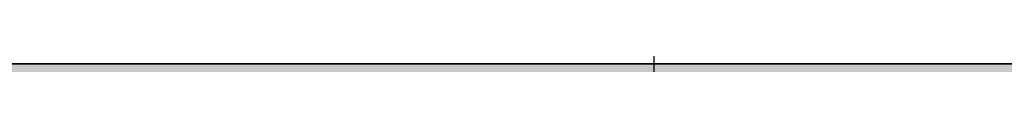
# Model space of a CAD drawing. Units: inches. Extents: x 2083 to 3317, y 1141 to 2115.
# Tile 51 of 256: x 2237.106 to 2238.294, y 1477.761 to 1477.761. Entities that reach past the tile are written whole.
import ezdxf

# ---------------------------------------------------------------- set-up
doc = ezdxf.new("R2010")
doc.units = ezdxf.units.IN
doc.layers.add('A-ANNO-DIMS', color=2, linetype='Continuous', lineweight=18)
doc.layers.add('A-WALL', color=7, linetype='Continuous', lineweight=35)
doc.layers.add('A-WALL-PATT', color=251, linetype='Continuous', lineweight=13, true_color=0x636466)
doc.styles.get("Standard").update_dxf_attribs({"font": 'arial.ttf'})
doc.dimstyles.new('ISO-25', dxfattribs={"dimtxt": 12, "dimasz": 12, "dimexe": 1.25, "dimexo": 0.625, "dimtad": 1, "dimlunit": 3, "dimtxsty": 'Standard', "dimcen": 2.5, "dimadec": 0, "dimazin": 0, "dimtfac": 1, "dimtmove": 0, "dimatfit": 3, "dimfxl": 1, "dimarcsym": 0})

# ---------------------------------------------------------------- blocks, each defined once
blk = doc.blocks.new('*D30')
at = {"layer": 'A-ANNO-DIMS', "color": 0, "lineweight": -2, "transparency": 16777216}
for p, q in [((2240.0179, 1445.2738), (2240.0179, 1448.0455)), ((2254.3293, 1445.2738), (2254.3293, 1448.0455)), ((2228.0179, 1446.7955), (2216.0179, 1446.7955)), ((2240.0179, 1446.7955), (2254.3293, 1446.7955)), ((2266.3293, 1446.7955), (2413.7649, 1446.7955))]:
    blk.add_line(p, q, dxfattribs=at)
at = {"layer": 'A-ANNO-DIMS', "color": 0, "transparency": 16777216}
for points in [[(2228.0179, 1448.7955), (2228.0179, 1444.7955), (2240.0179, 1446.7955)], [(2266.3293, 1448.7955), (2266.3293, 1444.7955), (2254.3293, 1446.7955)]]:
    blk.add_solid(points, dxfattribs=at)
at = {"layer": 'Defpoints', "color": 0, "transparency": 16777216}
for p in [(2254.3293, 1446.7955), (2240.0179, 1444.6488), (2254.3293, 1444.6488)]:
    blk.add_point(p, dxfattribs=at)
at = {"layer": 'A-ANNO-DIMS', "color": 0, "transparency": 16777216, "insert": (2346.0471, 1453.6252), "char_height": 12, "attachment_point": 5}
blk.add_mtext('WC 1\'-2 1/2" TYP.', dxfattribs=at)
blk = doc.blocks.new('*D31')
at = {"layer": 'A-ANNO-DIMS', "color": 0, "lineweight": -2, "transparency": 16777216}
for p, q in [((2237.8711, 1456.6488), (2237.8711, 1541.9152)), ((2239.3929, 1444.6488), (2236.6211, 1444.6488)), ((2237.8711, 1431.5475), (2237.8711, 1444.6488)), ((2239.3929, 1431.5475), (2236.6211, 1431.5475)), ((2237.8711, 1419.5475), (2237.8711, 1407.5475))]:
    blk.add_line(p, q, dxfattribs=at)
at = {"layer": 'A-ANNO-DIMS', "color": 0, "transparency": 16777216}
for points in [[(2235.8711, 1456.6488), (2239.8711, 1456.6488), (2237.8711, 1444.6488)], [(2235.8711, 1419.5475), (2239.8711, 1419.5475), (2237.8711, 1431.5475)]]:
    blk.add_solid(points, dxfattribs=at)
at = {"layer": 'Defpoints', "color": 0, "transparency": 16777216}
for p in [(2237.8711, 1444.6488), (2240.0179, 1444.6488), (2240.0179, 1431.5475)]:
    blk.add_point(p, dxfattribs=at)
at = {"layer": 'A-ANNO-DIMS', "color": 0, "transparency": 16777216, "insert": (2231.2175, 1505.282), "char_height": 12, "attachment_point": 5, "rotation": 90}
blk.add_mtext('1\'-1" TYP.', dxfattribs=at)
blk = doc.blocks.new('*D45')
at = {"layer": 'A-ANNO-DIMS', "color": 0, "lineweight": -2, "transparency": 16777216}
for p, q in [((2235.9598, 1478.3864), (2235.9598, 1531.3614)), ((2418.9598, 1478.3864), (2418.9598, 1531.3614)), ((2247.9598, 1530.1114), (2406.9598, 1530.1114))]:
    blk.add_line(p, q, dxfattribs=at)
at = {"layer": 'A-ANNO-DIMS', "color": 0, "transparency": 16777216}
for points in [[(2247.9598, 1532.1114), (2247.9598, 1528.1114), (2235.9598, 1530.1114)], [(2406.9598, 1532.1114), (2406.9598, 1528.1114), (2418.9598, 1530.1114)]]:
    blk.add_solid(points, dxfattribs=at)
at = {"layer": 'Defpoints', "color": 0, "transparency": 16777216}
for p in [(2418.9598, 1530.1114), (2235.9598, 1477.7614), (2418.9598, 1477.7614)]:
    blk.add_point(p, dxfattribs=at)
at = {"layer": 'A-ANNO-DIMS', "color": 0, "transparency": 16777216, "insert": (2327.4598, 1536.8673), "char_height": 12, "attachment_point": 5}
blk.add_mtext('15\'-3"', dxfattribs=at)
blk = doc.blocks.new('*D62')
at = {"layer": 'A-ANNO-DIMS', "color": 0, "lineweight": -2, "transparency": 16777216}
for p, q in [((2235.9598, 1469.3864), (2235.9598, 1522.3614)), ((2379.9598, 1469.3864), (2379.9598, 1522.3614)), ((2247.9598, 1521.1114), (2367.9598, 1521.1114))]:
    blk.add_line(p, q, dxfattribs=at)
at = {"layer": 'A-ANNO-DIMS', "color": 0, "transparency": 16777216}
for points in [[(2247.9598, 1523.1114), (2247.9598, 1519.1114), (2235.9598, 1521.1114)], [(2367.9598, 1523.1114), (2367.9598, 1519.1114), (2379.9598, 1521.1114)]]:
    blk.add_solid(points, dxfattribs=at)
at = {"layer": 'Defpoints', "color": 0, "transparency": 16777216}
for p in [(2379.9598, 1521.1114), (2235.9598, 1468.7614), (2379.9598, 1468.7614)]:
    blk.add_point(p, dxfattribs=at)
at = {"layer": 'A-ANNO-DIMS', "color": 0, "transparency": 16777216, "insert": (2307.9598, 1527.8632), "char_height": 12, "attachment_point": 5}
blk.add_mtext('12\'-0"', dxfattribs=at)

msp = doc.modelspace()

# ---------------------------------------------------------------- hatches: boundary and pattern name
at = {"layer": 'A-WALL-PATT'}
h = msp.add_hatch(color=256, dxfattribs=at)
h.dxf.hatch_style = 1
h.paths.add_polyline_path([(3126.9598, 2020.7614), (2748.9598, 2020.7614), (2604.9598, 2020.7614), (2226.9598, 2020.7614), (2226.9598, 1702.7614), (2466.9598, 1702.7614), (2466.9598, 1582.7614), (2418.9598, 1582.7614), (2418.9598, 1477.7614), (2226.9598, 1477.7614), (2226.9598, 1263.2614), (2544.9598, 1263.2614), (2544.9598, 1411.7614), (2604.9598, 1411.7614), (2685.9598, 1411.7614), (2685.9598, 1420.7614), (2604.9598, 1420.7614), (2604.9598, 1573.7614), (2604.9598, 1702.7614), (2604.9598, 2011.7614), (2748.9598, 2011.7614), (2748.9598, 1702.7614), (2862.9598, 1702.7614), (2862.9598, 1621.7614), (2871.9598, 1621.7614), (2871.9598, 1702.7614), (2883.9598, 1702.7614), (2883.9598, 1706.9395, -0.026459), (2883.9598, 1711.7614), (2757.9598, 1711.7614), (2757.9598, 1807.7614), (2787.9598, 1807.7614), (2787.9598, 1812.2614), (2757.9598, 1812.2614), (2757.9598, 2011.7614), (2877.9598, 2011.7614), (2877.9598, 1812.2614), (2847.9598, 1812.2614), (2847.9598, 1807.7614), (2889.8357, 1807.7614), (2889.8357, 1812.2614), (2882.4598, 1812.2614), (2882.4598, 2011.7614), (3117.9598, 2011.7614), (3117.9598, 1812.2614), (2937.8357, 1812.2614), (2937.8357, 1807.7614), (2995.7098, 1807.7614), (2995.7098, 1796.1177), (3000.2098, 1796.1177), (3000.2098, 1807.7614), (3117.9598, 1807.7614), (3117.9598, 1711.7614), (3000.2098, 1711.7614), (3000.2098, 1760.1177), (2998.5727, 1760.1177, -0.020711), (2995.7098, 1760.1177), (2995.7098, 1711.7614), (2931.9598, 1711.7614), (2931.9598, 1702.7614), (3126.9598, 1702.7614)])
h.paths.add_polyline_path([(2471.4598, 2011.7614), (2471.4598, 1810.0114), (2462.7169, 1810.0114), (2462.7169, 1805.5114), (2505.9598, 1805.5114), (2505.9598, 1810.0114), (2475.9598, 1810.0114), (2475.9598, 2011.7614), (2595.9598, 2011.7614), (2595.9598, 1810.0114), (2565.9598, 1810.0114), (2565.9598, 1805.5114), (2595.9598, 1805.5114), (2595.9598, 1711.7614), (2235.9598, 1711.7614), (2235.9598, 1805.5114), (2353.7098, 1805.5114), (2353.7098, 1796.0542), (2358.2098, 1796.0542), (2358.2098, 1805.5114), (2414.7169, 1805.5114), (2414.7169, 1810.0114), (2235.9598, 1810.0114), (2235.9598, 2011.7614)], flags=16)
h.paths.add_polyline_path([(2270.2047, 1994.61), (2270.2047, 1970.61), (2246.2047, 1970.61), (2246.2047, 1994.61)], flags=0)
edge = h.paths.add_edge_path(flags=0)
edge.add_ellipse((2332.0274, 1899.7982), major_axis=(-3.043, 3.043), ratio=0.168252, start_angle=-161.3322, end_angle=-156.3071, ccw=False)
edge.add_ellipse((2333.082, 1898.7435), major_axis=(-1.0546, 1.0546), ratio=0.453532, start_angle=-123.371, end_angle=-94.1591)
edge = h.paths.add_edge_path(flags=0)
edge.add_ellipse((2332.0274, 1968.8763), major_axis=(3.043, 3.043), ratio=0.168252, start_angle=18.6678, end_angle=23.6929)
edge.add_spline(control_points=[(2332.9256, 1970.6911), (2332.2268, 1970.3361), (2330.8937, 1969.6589), (2328.4131, 1970.9321), (2327.2039, 1967.7487), (2324.7096, 1969.9556), (2322.5328, 1967.0124), (2320.0128, 1971.2958), (2317.6803, 1968.1578), (2316.0405, 1967.102), (2315.4269, 1966.8096)], knot_values=[0, 0, 0, 0, 2.267059, 4.324559, 6.685584, 8.878641, 11.121502, 14.300359, 17.755284, 19.732645, 19.732645, 19.732645, 19.732645], degree=3, periodic=0)
edge.add_ellipse((2332.0274, 1968.8763), major_axis=(3.043, 3.043), ratio=0.168252, start_angle=18.6678, end_angle=23.6929, ccw=False)
edge.add_ellipse((2333.082, 1969.9309), major_axis=(1.0546, 1.0546), ratio=0.453532, start_angle=56.629, end_angle=85.8409, ccw=False)
edge = h.paths.add_edge_path(flags=0)
edge.add_spline(control_points=[(2296.4283, 1967.9879), (2293.6278, 1965.3363), (2287.7036, 1959.7271), (2299.7439, 1949.9957), (2294.5326, 1935.6685), (2290.5732, 1920.6035), (2293.3941, 1909.9737), (2296.1854, 1904.9665)], knot_values=[0.099185, 0.099185, 0.099185, 0.099185, 0.345301, 0.619822, 0.982653, 1.386093, 1.810555, 1.810555, 1.810555, 1.810555], degree=3, periodic=0)
edge.add_spline(control_points=[(2296.1854, 1904.9665), (2297.3836, 1902.6193), (2298.001, 1901.9493), (2298.553, 1901.4682)], knot_values=[0.006246, 0.006246, 0.006246, 0.006246, 0.055476, 0.055476, 0.055476, 0.055476], degree=3, periodic=0)
edge.add_spline(control_points=[(2298.553, 1901.4682), (2297.2586, 1900.9232), (2295.2253, 1900.2321), (2293.0602, 1900.6142), (2292.1014, 1900.7884), (2292.0896, 1900.7906)], knot_values=[0.312835, 0.312835, 0.312835, 0.312835, 0.40178, 0.474987, 0.475903, 0.475903, 0.475903, 0.475903], degree=3, periodic=0)
edge.add_arc((2292.7936, 1904.6641), 3.937, 215.4209, 259.6982, ccw=False)
edge.add_spline(control_points=[(2289.5853, 1902.3823), (2289.4767, 1902.5351), (2289.3685, 1902.688), (2289.2609, 1902.8412)], knot_values=[0.102872, 0.102872, 0.102872, 0.102872, 0.116896, 0.116896, 0.116896, 0.116896], degree=3, periodic=0)
edge.add_spline(control_points=[(2289.2609, 1902.8412), (2288.6866, 1902.5502), (2287.64, 1902.0199), (2285.8813, 1901.874), (2283.853, 1901.5044), (2281.72, 1899.7105), (2278.467, 1899.4929), (2276.1571, 1901.8832), (2272.259, 1899.8041), (2267.7776, 1901.8432), (2262.2439, 1900.184), (2257.4149, 1901.7821), (2254.3184, 1900.7261), (2253.1783, 1900.3373)], knot_values=[0, 0, 0, 0, 1.907977, 3.477176, 5.261074, 7.972851, 11.680248, 13.717921, 16.939592, 22.789562, 27.502503, 33.595215, 37.145618, 37.145618, 37.145618, 37.145618], degree=3, periodic=0)
edge.add_line((2253.1783, 1900.3373), (2250.2442, 1902.8412))
edge.add_line((2250.2442, 1902.8412), (2250.2442, 1965.8333))
edge.add_line((2250.2442, 1965.8333), (2253.1783, 1968.3371))
edge.add_spline(control_points=[(2253.1783, 1968.3371), (2254.3184, 1967.9483), (2257.4149, 1966.8924), (2262.2439, 1968.4904), (2267.7776, 1966.8313), (2271.5267, 1968.5372), (2273.8759, 1967.8283), (2274.2067, 1967.7276)], knot_values=[0, 0, 0, 0, 0.09018, 0.244935, 0.364644, 0.513233, 0.537855, 0.537855, 0.537855, 0.537855], degree=3, periodic=0)
edge.add_arc((2274.3529, 1963.7933), 3.937, 72.0511, 92.1279, ccw=False)
edge.add_arc((2281.2969, 1985.23), 18.5963, 252.05113, 288.56572)
edge.add_arc((2292.3167, 1956.0289), 12.6461, 71.02679, 113.77822, ccw=False)
edge = h.paths.add_edge_path(flags=0)
edge.add_spline(control_points=[(2274.8994, 1951.8562), (2275.0662, 1951.6166), (2275.2327, 1951.3766), (2275.398, 1951.1359)], knot_values=[1.409916, 1.409916, 1.409916, 1.409916, 1.43159, 1.43159, 1.43159, 1.43159], degree=3, periodic=0)
edge.add_spline(control_points=[(2275.398, 1951.1359), (2275.7921, 1950.5619), (2276.1792, 1949.9838), (2276.5455, 1949.3971)], knot_values=[1.358238, 1.358238, 1.358238, 1.358238, 1.409916, 1.409916, 1.409916, 1.409916], degree=3, periodic=0)
edge.add_line((2276.5455, 1949.3971), (2277.4373, 1947.8622))
edge.add_spline(control_points=[(2277.4373, 1947.8622), (2276.3038, 1945.6731), (2274.6397, 1942.4269), (2274.6316, 1938.0939), (2272.7991, 1930.8515), (2274.3564, 1943.897), (2275.9477, 1947.9234), (2276.5455, 1949.3971)], knot_values=[0.005632, 0.005632, 0.005632, 0.005632, 0.186014, 0.266002, 0.357087, 0.59639, 0.739732, 0.739732, 0.739732, 0.739732], degree=3, periodic=0)
edge.add_spline(control_points=[(2276.5455, 1949.3971), (2276.1792, 1949.9838), (2275.7921, 1950.5619), (2275.398, 1951.1359)], knot_values=[1.358238, 1.358238, 1.358238, 1.358238, 1.409916, 1.409916, 1.409916, 1.409916], degree=3, periodic=0)
edge.add_spline(control_points=[(2275.398, 1951.1359), (2274.9425, 1950.0805), (2274.2078, 1948.0253), (2273.9346, 1944.8515), (2272.4685, 1937.6275), (2273.4662, 1945.6965), (2274.7006, 1951.0595), (2274.8994, 1951.8562)], knot_values=[0.104364, 0.104364, 0.104364, 0.104364, 0.189636, 0.269624, 0.36071, 0.600013, 0.644622, 0.644622, 0.644622, 0.644622], degree=3, periodic=0)
h.paths.add_polyline_path([(2269.1675, 1963.1276, -0.357527), (2268.1706, 1960.9764, -0.092561), (2268.1706, 1939.4363, -0.357527), (2269.1675, 1937.2851, -0.357527), (2267.0163, 1938.282, -0.164785), (2254.6856, 1938.282, -0.357527), (2252.5344, 1937.2851, -0.357527), (2253.5313, 1939.4363, -0.092561), (2253.5313, 1960.9764, -0.357527), (2252.5344, 1963.1276, -0.357527), (2254.6856, 1962.1307, -0.164785), (2267.0163, 1962.1307, -0.357527)], flags=0)
h.paths.add_polyline_path([(2248.8741, 1967.8018), (2248.8741, 1957.0277), (2249.4578, 1957.0277), (2249.4578, 1911.6468), (2248.8741, 1911.6468), (2248.8741, 1900.8727), (2246.5119, 1900.8727, 0.197327), (2244.1497, 1902.4569), (2244.1497, 1966.2176, 0.197327), (2246.5119, 1967.8018)], flags=0)
h.paths.add_polyline_path([(2269.1675, 1931.3893, -0.357527), (2268.1706, 1929.2381, -0.092561), (2268.1706, 1907.6981, -0.357527), (2269.1675, 1905.5469, -0.357527), (2267.0163, 1906.5438, -0.164785), (2254.6856, 1906.5438, -0.357527), (2252.5344, 1905.5469, -0.357527), (2253.5313, 1907.6981, -0.092561), (2253.5313, 1929.2381, -0.357527), (2252.5344, 1931.3893, -0.357527), (2254.6856, 1930.3925, -0.164785), (2267.0163, 1930.3925, -0.357527)], flags=0)
edge = h.paths.add_edge_path(flags=0)
edge.add_spline(control_points=[(2276.1969, 1906.7237), (2276.1681, 1909.0289), (2276.114, 1913.3719), (2270.5984, 1924.925), (2273.9052, 1919.0128), (2275.9217, 1916.2621), (2275.4746, 1912.4021), (2277.2579, 1910.3806), (2276.696, 1908.225), (2276.6462, 1906.813), (2276.6178, 1906.0084)], knot_values=[0, 0, 0, 0, 8.61026, 16.221274, 18.843057, 23.804898, 27.440828, 29.356102, 31.203478, 33.650687, 33.650687, 33.650687, 33.650687], degree=3, periodic=0)
edge.add_spline(control_points=[(2276.6178, 1906.0084), (2276.6233, 1905.6241), (2276.4977, 1904.6287), (2275.4418, 1903.8547), (2274.9373, 1903.0804), (2274.8591, 1902.8412)], knot_values=[0.156488, 0.156488, 0.156488, 0.156488, 0.184398, 0.231376, 0.250598, 0.250598, 0.250598, 0.250598], degree=3, periodic=0)
edge.add_line((2274.8591, 1902.8412), (2276.506, 1902.8412))
edge.add_spline(control_points=[(2276.506, 1902.8412), (2276.7883, 1903.0849), (2277.6651, 1904.1252), (2278.2495, 1904.3407), (2277.6539, 1908.5274), (2278.1557, 1906.2278), (2278.1005, 1905.2859), (2278.8467, 1904.069), (2277.8568, 1903.4149), (2277.8742, 1902.991), (2277.9036, 1902.8412)], knot_values=[0.059574, 0.059574, 0.059574, 0.059574, 0.080753, 0.103741, 0.16972, 0.176036, 0.207137, 0.240474, 0.262341, 0.27366, 0.27366, 0.27366, 0.27366], degree=3, periodic=0)
edge.add_line((2277.9036, 1902.8412), (2280.0298, 1902.8412))
edge.add_spline(control_points=[(2280.0298, 1902.8412), (2279.8882, 1903.0884), (2279.4993, 1903.9816), (2280.1523, 1905.9393), (2278.1036, 1909.6578), (2279.7624, 1907.1853), (2280.3279, 1904.8749), (2280.4851, 1903.4896), (2281.4633, 1903.2494), (2281.7583, 1902.9365), (2281.834, 1902.8412)], knot_values=[0.013856, 0.013856, 0.013856, 0.013856, 0.034874, 0.088867, 0.107879, 0.126738, 0.158714, 0.193757, 0.217487, 0.226722, 0.226722, 0.226722, 0.226722], degree=3, periodic=0)
edge.add_spline(control_points=[(2281.834, 1902.8412), (2281.7875, 1902.8267), (2281.647, 1902.783), (2281.3955, 1902.8595), (2281.0881, 1902.9852), (2280.7207, 1903.0609), (2280.3335, 1903.0257), (2280.1248, 1902.8989), (2280.0298, 1902.8412)], knot_values=[0, 0, 0, 0, 0.14413, 0.435517, 0.749276, 1.153046, 1.548371, 1.878348, 1.878348, 1.878348, 1.878348], degree=3, periodic=0)
edge.add_line((2280.0298, 1902.8412), (2277.9036, 1902.8412))
edge.add_spline(control_points=[(2277.9036, 1902.8412), (2277.8929, 1902.7959), (2277.8654, 1902.6796), (2277.6075, 1902.6875), (2277.2741, 1902.8007), (2276.8379, 1902.6198), (2276.5838, 1902.7893), (2276.506, 1902.8412)], knot_values=[0, 0, 0, 0, 0.127189, 0.326199, 0.628009, 1.24357, 1.515331, 1.515331, 1.515331, 1.515331], degree=3, periodic=0)
edge.add_line((2276.506, 1902.8412), (2274.8591, 1902.8412))
edge.add_spline(control_points=[(2274.8591, 1902.8412), (2274.8144, 1902.8986), (2274.7251, 1903.0134), (2274.4935, 1903.119), (2274.2443, 1902.9605), (2273.9371, 1903.1849), (2273.614, 1902.9831), (2273.4083, 1902.883), (2273.3223, 1902.8412)], knot_values=[0, 0, 0, 0, 0.21843, 0.436957, 0.687977, 0.990379, 1.398396, 1.69185, 1.69185, 1.69185, 1.69185], degree=3, periodic=0)
edge.add_spline(control_points=[(2273.3223, 1902.8412), (2273.6167, 1903.4457), (2274.274, 1904.5383), (2276.0272, 1904.5737), (2276.207, 1906.5836), (2276.1969, 1906.7237)], knot_values=[0.012227, 0.012227, 0.012227, 0.012227, 0.059472, 0.106218, 0.134458, 0.134458, 0.134458, 0.134458], degree=3, periodic=0)
h.paths.add_polyline_path([(2270.7761, 1897.7898), (2270.7761, 1873.7898), (2246.7761, 1873.7898), (2246.7761, 1897.7898)], flags=0)
h.paths.add_polyline_path([(2353.7098, 1760.0051), (2353.7098, 1760.0542), (2358.2098, 1760.0542, -0.033729)], flags=0)
h.paths.add_polyline_path([(2321.8191, 1737.5292), (2341.9953, 1737.5292, -0.414214), (2343.2033, 1736.3212), (2343.2033, 1721.0206, -0.414214), (2341.9953, 1719.8127), (2321.8191, 1719.8127, -0.414214), (2320.6112, 1721.0206), (2320.6112, 1736.3212, -0.414214)], flags=0)
h.paths.add_polyline_path([(2324.235, 1736.3212), (2339.5794, 1736.3212, -0.414214), (2341.9953, 1733.9053), (2341.9953, 1725.4497, -0.414214), (2339.5794, 1723.0338), (2333.6806, 1723.0338), (2333.8453, 1722.0455, -0.870646), (2335.4254, 1721.8259, -0.767327), (2333.9227, 1721.4232), (2331.291, 1721.4232, -0.767327), (2329.7883, 1721.8259, -0.870646), (2331.3684, 1722.0455), (2331.5331, 1723.0338), (2324.235, 1723.0338, -0.414214), (2321.8191, 1725.4497), (2321.8191, 1733.9053, -0.414214)], flags=0)
h.paths.add_polyline_path([(2570.4838, 1928.6154), (2589.6838, 1928.6154), (2590.1688, 1928.6154), (2590.1688, 1904.9934), (2570.4838, 1904.9934)], flags=0)
h.paths.add_polyline_path([(2574.4473, 1927.2638, -1), (2572.8288, 1927.2638, -1)], flags=0)
h.paths.add_polyline_path([(2573.0899, 1926.9409), (2573.925, 1927.776), (2574.1477, 1927.5533), (2573.3126, 1926.7182)], flags=0)
h.paths.add_polyline_path([(2578.7791, 1919.7296, -1), (2571.5917, 1919.7296, -1)], flags=0)
h.paths.add_polyline_path([(2578.3854, 1919.7296, -1), (2571.9854, 1919.7296, -1)], flags=0)
h.paths.add_polyline_path([(2331.5958, 1729.4762, -1), (2333.618, 1729.4762, -1)], flags=0)
h.paths.add_polyline_path([(2578.0342, 1927.2638, -1), (2576.4157, 1927.2638, -1)], flags=0)
h.paths.add_polyline_path([(2576.6889, 1927.5311), (2576.9116, 1927.7538), (2577.7467, 1926.9186), (2577.524, 1926.6959)], flags=0)
h.paths.add_polyline_path([(2578.1391, 1909.8595, -1), (2572.2317, 1909.8595, -1)], flags=0)
h.paths.add_polyline_path([(2577.7454, 1909.8595, -1), (2572.6254, 1909.8595, -1)], flags=0)
h.paths.add_polyline_path([(2583.7977, 1927.2638, -1), (2582.1792, 1927.2638, -1)], flags=0)
h.paths.add_polyline_path([(2582.7186, 1927.7538), (2583.5538, 1926.9186), (2583.3311, 1926.6959), (2582.4959, 1927.5311)], flags=0)
h.paths.add_polyline_path([(2582.4959, 1927.5311), (2582.7186, 1927.7538), (2583.5538, 1926.9186), (2583.3311, 1926.6959)], flags=0)
h.paths.add_polyline_path([(2587.7391, 1920.5296, -1), (2581.8317, 1920.5296, -1)], flags=0)
h.paths.add_polyline_path([(2587.3454, 1920.5296, -1), (2582.2254, 1920.5296, -1)], flags=0)
h.paths.add_polyline_path([(2587.3846, 1927.2638, -1), (2585.7661, 1927.2638, -1)], flags=0)
h.paths.add_polyline_path([(2586.082, 1926.9802), (2586.9172, 1927.8154), (2587.1399, 1927.5927), (2586.3047, 1926.7575)], flags=0)
h.paths.add_polyline_path([(2588.3791, 1910.6595, -1), (2581.1917, 1910.6595, -1)], flags=0)
h.paths.add_polyline_path([(2587.9854, 1910.6595, -1), (2581.5854, 1910.6595, -1)], flags=0)
h.paths.add_polyline_path([(2417.1677, 1729.4779), (2437.3439, 1729.4779, -0.414214), (2438.5519, 1728.2699), (2438.5519, 1712.9693, -0.414214), (2437.3439, 1711.7614), (2417.1677, 1711.7614, -0.414214), (2415.9598, 1712.9693), (2415.9598, 1728.2699, -0.414214)], flags=0)
h.paths.add_polyline_path([(2419.5836, 1728.2699), (2434.928, 1728.2699, -0.414214), (2437.3439, 1725.8541), (2437.3439, 1717.3984, -0.414214), (2434.928, 1714.9825), (2429.0292, 1714.9825), (2429.1939, 1713.9942, -0.870646), (2430.774, 1713.7746, -0.767327), (2429.2713, 1713.372), (2426.6396, 1713.372, -0.767327), (2425.1369, 1713.7746, -0.870646), (2426.717, 1713.9942), (2426.8817, 1714.9825), (2419.5836, 1714.9825, -0.414214), (2417.1677, 1717.3984), (2417.1677, 1725.8541, -0.414214)], flags=0)
h.paths.add_polyline_path([(2419.5836, 1728.2699), (2434.928, 1728.2699, -0.414214), (2437.3439, 1725.8541), (2437.3439, 1717.3984, -0.414214), (2434.928, 1714.9825), (2429.0292, 1714.9825), (2428.3581, 1719.009), (2427.5528, 1719.009), (2426.8817, 1714.9825), (2419.5836, 1714.9825, -0.414214), (2417.1677, 1717.3984), (2417.1677, 1725.8541, -0.414214)], flags=0)
h.paths.add_polyline_path([(2426.9444, 1721.4249, -1), (2428.9666, 1721.4249, -1)], flags=0)
h.paths.add_polyline_path([(2475.9598, 1702.7614), (2595.9598, 1702.7614), (2595.9598, 1582.7614), (2475.9598, 1582.7614)], flags=16)
h.paths.add_polyline_path([(2427.9598, 1573.7614), (2595.9598, 1573.7614), (2595.9598, 1468.7614), (2595.9598, 1420.7614), (2384.4598, 1420.7614), (2384.4598, 1468.7614), (2427.9598, 1468.7614)], flags=16)
h.paths.add_polyline_path([(2379.9598, 1468.7614), (2379.9598, 1420.7614), (2235.9598, 1420.7614), (2235.9598, 1468.7614)], flags=16)
h.paths.add_polyline_path([(2317.816, 1466.6958), (2337.9922, 1466.6958, -0.414214), (2339.2002, 1465.4878), (2339.2002, 1450.1872, -0.414214), (2337.9922, 1448.9792), (2317.816, 1448.9792, -0.414214), (2316.6081, 1450.1872), (2316.6081, 1465.4878, -0.414214)], flags=0)
h.paths.add_polyline_path([(2320.2319, 1465.4878), (2335.5763, 1465.4878, -0.414214), (2337.9922, 1463.0719), (2337.9922, 1454.6163, -0.414214), (2335.5763, 1452.2004), (2329.6775, 1452.2004), (2329.8422, 1451.212, -0.870646), (2331.4223, 1450.9925, -0.767327), (2329.9196, 1450.5898), (2327.2879, 1450.5898, -0.767327), (2325.7852, 1450.9925, -0.870646), (2327.3653, 1451.212), (2327.53, 1452.2004), (2320.2319, 1452.2004, -0.414214), (2317.816, 1454.6163), (2317.816, 1463.0719, -0.414214)], flags=0)
h.paths.add_polyline_path([(2320.2319, 1465.4878), (2335.5763, 1465.4878, -0.414214), (2337.9922, 1463.0719), (2337.9922, 1454.6163, -0.414214), (2335.5763, 1452.2004), (2329.6775, 1452.2004), (2329.0064, 1456.2269), (2328.2011, 1456.2269), (2327.53, 1452.2004), (2320.2319, 1452.2004, -0.414214), (2317.816, 1454.6163), (2317.816, 1463.0719, -0.414214)], flags=0)
h.paths.add_polyline_path([(2327.5926, 1458.6428, -1), (2329.6148, 1458.6428, -1)], flags=0)
h.paths.add_polyline_path([(2244.4117, 1433.3405), (2241.9209, 1433.3405, -0.414214), (2240.0179, 1435.2435), (2240.0179, 1440.9528, -0.414211), (2241.9209, 1442.8559), (2244.4117, 1442.8559, -1.976472)], flags=0)
h.paths.add_polyline_path([(2245.3569, 1434.3975, -0.414214), (2245.3569, 1441.7988, -2.144098)], flags=0)
h.paths.add_polyline_path([(2535.9598, 1416.2614), (2535.9598, 1272.2614), (2235.9598, 1272.2614), (2235.9598, 1416.2614)], flags=16)
h.paths.add_polyline_path([(2260.1196, 1384.2928), (2260.1196, 1362.0386), (2237.8654, 1362.0386), (2237.8654, 1384.2928)], flags=0)
edge = h.paths.add_edge_path(flags=0)
edge.add_line((2318.2518, 1362.0933), (2318.1458, 1362.001))
edge.add_ellipse((2317.4451, 1360.431), major_axis=(2.8216, 2.8216), ratio=0.168252, start_angle=18.6678, end_angle=20.9481, ccw=False)
edge.add_ellipse((2318.423, 1361.409), major_axis=(0.9779, 0.9779), ratio=0.453532, start_angle=56.629, end_angle=70.2262, ccw=False)
edge = h.paths.add_edge_path(flags=0)
edge.add_line((2319.1074, 1295.5711), (2319.015, 1295.6771))
edge.add_ellipse((2317.4451, 1296.3778), major_axis=(-2.8216, 2.8216), ratio=0.168252, start_angle=-161.3322, end_angle=-159.0519, ccw=False)
edge.add_ellipse((2318.423, 1295.3999), major_axis=(-0.9779, 0.9779), ratio=0.453532, start_angle=-123.371, end_angle=-109.7738)
edge = h.paths.add_edge_path(flags=0)
edge.add_spline(control_points=[(2284.2103, 1301.1702), (2284.5807, 1300.4447), (2284.8912, 1299.892), (2285.1596, 1299.461)], knot_values=[0.039066, 0.039066, 0.039066, 0.039066, 0.055476, 0.055476, 0.055476, 0.055476], degree=3, periodic=0)
edge.add_line((2285.1596, 1299.461), (2284.2103, 1301.1702))
edge = h.paths.add_edge_path(flags=0)
edge.add_line((2280.4125, 1297.298), (2283.37, 1297.0361))
edge.add_line((2283.37, 1297.0361), (2286.4057, 1297.9263))
edge.add_spline(control_points=[(2286.4057, 1297.9263), (2285.3055, 1297.4631), (2284.3448, 1297.1292), (2283.37, 1297.0361)], knot_values=[0.394369, 0.394369, 0.394369, 0.394369, 0.475903, 0.475903, 0.475903, 0.475903], degree=3, periodic=0)
edge.add_spline(control_points=[(2283.37, 1297.0361), (2283.2814, 1297.0277), (2282.3163, 1296.9573), (2281.3125, 1297.1345), (2280.4234, 1297.296), (2280.4125, 1297.298)], knot_values=[0.312835, 0.312835, 0.312835, 0.312835, 0.320246, 0.393453, 0.394369, 0.394369, 0.394369, 0.394369], degree=3, periodic=0)
edge = h.paths.add_edge_path(flags=0)
edge.add_line((2284.4356, 1359.6073), (2280.4463, 1355.328))
edge.add_line((2280.4463, 1355.328), (2279.58, 1351.0178))
edge.add_line((2279.58, 1351.0178), (2282.413, 1346.5804))
edge.add_spline(control_points=[(2282.413, 1346.5804), (2283.1533, 1345.5892), (2284.2529, 1344.0289), (2284.801, 1342.3872), (2284.9352, 1341.8055)], knot_values=[1.240098, 1.240098, 1.240098, 1.240098, 1.332892, 1.382712, 1.382712, 1.382712, 1.382712], degree=3, periodic=0)
edge.add_spline(control_points=[(2284.9352, 1341.8055), (2285.3191, 1340.1406), (2285.233, 1338.4092), (2284.9099, 1336.6541)], knot_values=[1.097484, 1.097484, 1.097484, 1.097484, 1.240098, 1.240098, 1.240098, 1.240098], degree=3, periodic=0)
edge.add_spline(control_points=[(2284.9099, 1336.6541), (2284.5868, 1334.899), (2284.0267, 1333.1203), (2283.4626, 1331.3606)], knot_values=[0.95487, 0.95487, 0.95487, 0.95487, 1.097484, 1.097484, 1.097484, 1.097484], degree=3, periodic=0)
edge.add_line((2283.4626, 1331.3606), (2281.8904, 1326.1534))
edge.add_line((2281.8904, 1326.1534), (2280.7563, 1321.0561))
edge.add_line((2280.7563, 1321.0561), (2280.2992, 1316.002))
edge.add_line((2280.2992, 1316.002), (2280.7159, 1310.9501))
edge.add_line((2280.7159, 1310.9501), (2282.0281, 1305.9721))
edge.add_line((2282.0281, 1305.9721), (2284.2103, 1301.1702))
edge.add_spline(control_points=[(2284.2103, 1301.1702), (2283.3407, 1302.7302), (2282.6119, 1304.3365), (2282.0281, 1305.9721)], knot_values=[0.099185, 0.099185, 0.099185, 0.099185, 0.241799, 0.241799, 0.241799, 0.241799], degree=3, periodic=0)
edge.add_spline(control_points=[(2282.0281, 1305.9721), (2281.4443, 1307.6078), (2281.0055, 1309.2728), (2280.7159, 1310.9501)], knot_values=[0.241799, 0.241799, 0.241799, 0.241799, 0.384413, 0.384413, 0.384413, 0.384413], degree=3, periodic=0)
edge.add_spline(control_points=[(2280.7159, 1310.9501), (2280.4332, 1312.5876), (2280.2894, 1314.277), (2280.2989, 1315.962), (2280.2992, 1316.002)], knot_values=[0.384413, 0.384413, 0.384413, 0.384413, 0.523647, 0.527028, 0.527028, 0.527028, 0.527028], degree=3, periodic=0)
edge.add_spline(control_points=[(2280.2992, 1316.002), (2280.3123, 1317.687), (2280.4779, 1319.3679), (2280.7563, 1321.0561)], knot_values=[0.527028, 0.527028, 0.527028, 0.527028, 0.669642, 0.669642, 0.669642, 0.669642], degree=3, periodic=0)
edge.add_spline(control_points=[(2280.7563, 1321.0561), (2281.0346, 1322.7443), (2281.4259, 1324.4396), (2281.8904, 1326.1534)], knot_values=[0.669642, 0.669642, 0.669642, 0.669642, 0.812256, 0.812256, 0.812256, 0.812256], degree=3, periodic=0)
edge.add_spline(control_points=[(2281.8904, 1326.1534), (2282.2644, 1327.5333), (2282.7879, 1329.2618), (2283.3528, 1331.0178), (2283.4626, 1331.3606)], knot_values=[0.812256, 0.812256, 0.812256, 0.812256, 0.927087, 0.95487, 0.95487, 0.95487, 0.95487], degree=3, periodic=0)
edge.add_line((2283.4626, 1331.3606), (2284.9099, 1336.6541))
edge.add_line((2284.9099, 1336.6541), (2284.9352, 1341.8055))
edge.add_line((2284.9352, 1341.8055), (2282.413, 1346.5804))
edge.add_spline(control_points=[(2282.413, 1346.5804), (2281.2751, 1348.1038), (2280.0784, 1349.5703), (2279.58, 1351.0178)], knot_values=[1.382712, 1.382712, 1.382712, 1.382712, 1.525326, 1.525326, 1.525326, 1.525326], degree=3, periodic=0)
edge.add_spline(control_points=[(2279.58, 1351.0178), (2279.4433, 1351.4147), (2279.1363, 1352.8569), (2279.7352, 1354.2904), (2280.4463, 1355.328)], knot_values=[1.525326, 1.525326, 1.525326, 1.525326, 1.564439, 1.667941, 1.667941, 1.667941, 1.667941], degree=3, periodic=0)
edge.add_spline(control_points=[(2280.4463, 1355.328), (2281.4261, 1356.7578), (2282.9308, 1358.1826), (2284.4356, 1359.6073)], knot_values=[1.667941, 1.667941, 1.667941, 1.667941, 1.810555, 1.810555, 1.810555, 1.810555], degree=3, periodic=0)
edge.add_arc((2280.6231, 1348.5182), 11.7262, 71.02679, 113.77822)
edge.add_arc((2270.4049, 1375.5952), 17.2436, 252.05113, 288.56572, ccw=False)
edge.add_arc((2263.966, 1355.7178), 3.6506, 72.0511, 92.1279)
edge.add_arc((2263.966, 1355.7178), 3.6506, 92.1279, 177.9851)
edge.add_spline(control_points=[(2260.3176, 1355.8462), (2260.2604, 1354.2207), (2260.5513, 1350.1865), (2262.9993, 1346.7663), (2264.4727, 1344.649)], knot_values=[1.43159, 1.43159, 1.43159, 1.43159, 1.564144, 1.770695, 1.770695, 1.770695, 1.770695], degree=3, periodic=0)
edge.add_line((2264.4727, 1344.649), (2264.9356, 1343.9825))
edge.add_spline(control_points=[(2263.801, 1340.2481), (2263.8432, 1340.5141), (2264.0672, 1341.7565), (2264.5127, 1343.0025), (2264.935, 1343.9811)], knot_values=[0.53657, 0.53657, 0.53657, 0.53657, 0.559349, 0.644622, 0.644622, 0.644622, 0.644622], degree=3, periodic=0)
edge.add_spline(control_points=[(2264.935, 1343.9811), (2265.1178, 1343.715), (2265.2989, 1343.4479), (2265.4768, 1343.1794)], knot_values=[1.384077, 1.384077, 1.384077, 1.384077, 1.409916, 1.409916, 1.409916, 1.409916], degree=3, periodic=0)
edge.add_spline(control_points=[(2265.4768, 1343.1794), (2265.6546, 1342.9108), (2265.8293, 1342.6408), (2265.9991, 1342.3688)], knot_values=[1.358238, 1.358238, 1.358238, 1.358238, 1.384077, 1.384077, 1.384077, 1.384077], degree=3, periodic=0)
edge.add_line((2265.9991, 1342.3688), (2266.826, 1340.9455))
edge.add_spline(control_points=[(2266.826, 1340.9455), (2268.8944, 1337.0897), (2271.3982, 1325.843), (2270.5162, 1310.5686), (2275.9194, 1301.8606), (2277.7895, 1299.1994)], knot_values=[0.116896, 0.116896, 0.116896, 0.116896, 0.472987, 1.050969, 1.313793, 1.313793, 1.313793, 1.313793], degree=3, periodic=0)
edge.add_spline(control_points=[(2277.7895, 1299.1994), (2277.8394, 1299.1285), (2277.8894, 1299.0575), (2277.9396, 1298.9866)], knot_values=[0.109884, 0.109884, 0.109884, 0.109884, 0.116896, 0.116896, 0.116896, 0.116896], degree=3, periodic=0)
edge.add_line((2277.9396, 1298.9866), (2277.7888, 1299.1991))
edge.add_spline(control_points=[(2277.7888, 1299.1991), (2277.2566, 1298.9294), (2276.2864, 1298.4379), (2275.0394, 1298.3344), (2274.3833, 1298.2389), (2274.2153, 1298.2093)], knot_values=[33.12187, 33.12187, 33.12187, 33.12187, 35.029056, 36.598255, 37.144827, 37.144827, 37.144827, 37.144827], degree=3, periodic=0)
edge.add_line((2274.2153, 1298.2093), (2273.0731, 1297.893))
edge.add_spline(control_points=[(2273.0731, 1297.893), (2272.3229, 1297.5798), (2271.0392, 1296.5105), (2269.2484, 1296.2261), (2268.4231, 1296.3747)], knot_values=[26.532584, 26.532584, 26.532584, 26.532584, 29.198919, 31.839101, 31.839101, 31.839101, 31.839101], degree=3, periodic=0)
edge.add_line((2268.4231, 1296.3747), (2263.8785, 1297.4575))
edge.add_spline(control_points=[(2263.8785, 1297.4575), (2263.5561, 1297.3594), (2261.8603, 1296.8387), (2260.2388, 1297.2824), (2258.9335, 1297.5165)], knot_values=[15.919551, 15.919551, 15.919551, 15.919551, 16.939592, 21.226067, 21.226067, 21.226067, 21.226067], degree=3, periodic=0)
edge.add_line((2258.9335, 1297.5165), (2254.0552, 1297.329))
edge.add_spline(control_points=[(2254.0552, 1297.329), (2253.7555, 1297.2958), (2252.1137, 1297.1652), (2250.4619, 1297.5442), (2249.1297, 1297.6679)], knot_values=[5.306517, 5.306517, 5.306517, 5.306517, 6.276435, 10.613034, 10.613034, 10.613034, 10.613034], degree=3, periodic=0)
edge.add_line((2249.1297, 1297.6679), (2244.3316, 1296.8778))
edge.add_line((2244.3316, 1296.8778), (2241.611, 1299.1994))
edge.add_line((2241.611, 1299.1994), (2241.611, 1357.6094))
edge.add_line((2241.611, 1357.6094), (2244.3316, 1359.9311))
edge.add_line((2244.3316, 1359.9311), (2252.7288, 1359.5427))
edge.add_spline(control_points=[(2252.7288, 1359.5427), (2252.8709, 1359.5464), (2253.3057, 1359.5482), (2253.7398, 1359.5143), (2254.0317, 1359.4824)], knot_values=[0.233291, 0.233291, 0.233291, 0.233291, 0.244935, 0.268927, 0.268927, 0.268927, 0.268927], degree=3, periodic=0)
edge.add_line((2254.0317, 1359.4824), (2259.5872, 1359.4164))
edge.add_spline(control_points=[(2259.5872, 1359.4164), (2260.6771, 1359.6285), (2262.0732, 1359.897), (2263.5237, 1359.4593), (2263.8304, 1359.366)], knot_values=[0.422516, 0.422516, 0.422516, 0.422516, 0.513233, 0.537855, 0.537855, 0.537855, 0.537855], degree=3, periodic=0)
edge.add_arc((2263.966, 1355.7178), 3.6506, 72.0511, 92.1279, ccw=False)
edge.add_arc((2270.4049, 1375.5952), 17.2436, 252.05113, 288.56572)
edge.add_arc((2280.6231, 1348.5182), 11.7262, 71.02679, 113.77822, ccw=False)
h.paths.add_polyline_path([(2240.3405, 1359.4347), (2240.3405, 1349.4444), (2240.8818, 1349.4444), (2240.8818, 1307.3645), (2240.3405, 1307.3645), (2240.3405, 1297.3741), (2238.1502, 1297.3741, 0.197327), (2235.9598, 1298.8431), (2235.9598, 1357.9657, 0.197327), (2238.1502, 1359.4347)], flags=0)
h.paths.add_polyline_path([(2259.1578, 1355.1005, -0.357527), (2258.2334, 1353.1058, -0.092561), (2258.2334, 1333.1326, -0.357527), (2259.1578, 1331.1379, -0.357527), (2257.1631, 1332.0622, -0.164785), (2245.7293, 1332.0622, -0.357527), (2243.7346, 1331.1379, -0.357527), (2244.6589, 1333.1326, -0.092561), (2244.6589, 1353.1058, -0.357527), (2243.7346, 1355.1005, -0.357527), (2245.7293, 1354.1761, -0.164785), (2257.1631, 1354.1761, -0.357527)], flags=0)
edge = h.paths.add_edge_path(flags=0)
edge.add_line((2265.9991, 1342.3688), (2266.826, 1340.9455))
edge.add_line((2266.826, 1340.9455), (2265.3076, 1337.8141))
edge.add_line((2265.3076, 1337.8141), (2264.3582, 1334.6529))
edge.add_line((2264.3582, 1334.6529), (2264.262, 1333.7997))
edge.add_spline(control_points=[(2264.262, 1333.7997), (2264.2084, 1333.1871), (2264.1621, 1332.3655), (2264.0071, 1331.4139), (2263.969, 1331.2018)], knot_values=[0.464444, 0.464444, 0.464444, 0.464444, 0.516691, 0.531608, 0.531608, 0.531608, 0.531608], degree=3, periodic=0)
edge.add_spline(control_points=[(2263.969, 1331.2018), (2263.7745, 1330.1189), (2263.4244, 1328.7908), (2263.2574, 1328.5307), (2263.234, 1328.5146)], knot_values=[0.372682, 0.372682, 0.372682, 0.372682, 0.44885, 0.464444, 0.464444, 0.464444, 0.464444], degree=3, periodic=0)
edge.add_spline(control_points=[(2263.234, 1328.5146), (2263.0964, 1328.4202), (2263.1312, 1329.3015), (2263.275, 1330.6157)], knot_values=[0.280919, 0.280919, 0.280919, 0.280919, 0.372682, 0.372682, 0.372682, 0.372682], degree=3, periodic=0)
edge.add_spline(control_points=[(2263.275, 1330.6157), (2263.4187, 1331.93), (2263.6715, 1333.6773), (2263.9699, 1335.315)], knot_values=[0.189157, 0.189157, 0.189157, 0.189157, 0.280919, 0.280919, 0.280919, 0.280919], degree=3, periodic=0)
edge.add_spline(control_points=[(2263.9699, 1335.315), (2264.1005, 1336.0322), (2264.4188, 1337.6219), (2264.7548, 1338.8644), (2264.9474, 1339.4911)], knot_values=[0.097394, 0.097394, 0.097394, 0.097394, 0.137578, 0.189157, 0.189157, 0.189157, 0.189157], degree=3, periodic=0)
edge.add_spline(control_points=[(2264.9474, 1339.4911), (2265.29, 1340.6061), (2265.6442, 1341.494), (2265.9991, 1342.3688)], knot_values=[0.005632, 0.005632, 0.005632, 0.005632, 0.097394, 0.097394, 0.097394, 0.097394], degree=3, periodic=0)
h.paths.add_polyline_path([(2259.1578, 1325.671, -0.357527), (2258.2334, 1323.6763, -0.092561), (2258.2334, 1303.7031, -0.357527), (2259.1578, 1301.7084, -0.357527), (2257.1631, 1302.6327, -0.164785), (2245.7293, 1302.6327, -0.357527), (2243.7346, 1301.7084, -0.357527), (2244.6589, 1303.7031, -0.092561), (2244.6589, 1323.6763, -0.357527), (2243.7346, 1325.671, -0.357527), (2245.7293, 1324.7466, -0.164785), (2257.1631, 1324.7466, -0.357527)], flags=0)
edge = h.paths.add_edge_path(flags=0)
edge.add_spline(control_points=[(2261.7089, 1317.3114), (2261.6795, 1317.4176), (2261.7619, 1317.3885), (2262.4907, 1316.0899), (2262.9622, 1315.3009)], knot_values=[14.955861, 14.955861, 14.955861, 14.955861, 16.221274, 18.694826, 18.694826, 18.694826, 18.694826], degree=3, periodic=0)
edge.add_spline(control_points=[(2262.9622, 1315.3009), (2262.9904, 1315.2536), (2263.7021, 1314.0674), (2264.349, 1313.1272), (2264.7301, 1312.1642)], knot_values=[18.694826, 18.694826, 18.694826, 18.694826, 18.843057, 22.433791, 22.433791, 22.433791, 22.433791], degree=3, periodic=0)
edge.add_spline(control_points=[(2264.7301, 1312.1642), (2264.8756, 1311.7964), (2265.1769, 1310.7698), (2265.1431, 1309.5593), (2265.2477, 1308.8242)], knot_values=[22.433791, 22.433791, 22.433791, 22.433791, 23.804898, 26.172756, 26.172756, 26.172756, 26.172756], degree=3, periodic=0)
edge.add_line((2265.2477, 1308.8242), (2265.8508, 1307.1719))
edge.add_spline(control_points=[(2265.8508, 1307.1719), (2266.065, 1306.8217), (2266.3844, 1306.3322), (2266.4244, 1305.7805), (2266.4204, 1305.6112)], knot_values=[28.062562, 28.062562, 28.062562, 28.062562, 29.356102, 29.911721, 29.911721, 29.911721, 29.911721], degree=3, periodic=0)
edge.add_spline(control_points=[(2266.4204, 1305.6112), (2266.4161, 1305.4326), (2266.394, 1305.25), (2266.3648, 1305.0659)], knot_values=[29.911721, 29.911721, 29.911721, 29.911721, 30.497837, 30.497837, 30.497837, 30.497837], degree=3, periodic=0)
edge.add_line((2266.3648, 1305.0659), (2266.0662, 1302.1363))
edge.add_spline(control_points=[(2266.0662, 1302.1363), (2266.0712, 1301.78), (2265.9981, 1301.2), (2265.6633, 1300.759), (2265.5089, 1300.5859)], knot_values=[0.156488, 0.156488, 0.156488, 0.156488, 0.184398, 0.203543, 0.203543, 0.203543, 0.203543], degree=3, periodic=0)
edge.add_line((2265.5089, 1300.5859), (2264.4353, 1299.1994))
edge.add_line((2264.4353, 1299.1994), (2265.9624, 1299.1994))
edge.add_line((2265.9624, 1299.1994), (2267.336, 1301.1753))
edge.add_line((2267.336, 1301.1753), (2267.3117, 1301.9862))
edge.add_spline(control_points=[(2267.3117, 1301.9862), (2267.2611, 1302.8624), (2267.1602, 1303.7371), (2267.2715, 1303.3259)], knot_values=[0.126229, 0.126229, 0.126229, 0.126229, 0.166617, 0.166617, 0.166617, 0.166617], degree=3, periodic=0)
edge.add_spline(control_points=[(2267.2715, 1303.3259), (2267.28, 1303.2943), (2267.3098, 1303.1754), (2267.3735, 1302.8836), (2267.4061, 1302.6828), (2267.4179, 1302.601)], knot_values=[0.166617, 0.166617, 0.166617, 0.166617, 0.16972, 0.176036, 0.180765, 0.180765, 0.180765, 0.180765], degree=3, periodic=0)
edge.add_spline(control_points=[(2267.7439, 1300.9875), (2267.6876, 1301.1509), (2267.4805, 1301.6567), (2267.4838, 1302.1448), (2267.4179, 1302.601)], knot_values=[0.180765, 0.180765, 0.180765, 0.180765, 0.193767, 0.220139, 0.220139, 0.220139, 0.220139], degree=3, periodic=0)
edge.add_line((2267.4179, 1302.601), (2267.7439, 1300.9875))
edge.add_spline(control_points=[(2267.7439, 1300.9875), (2267.832, 1300.7319), (2267.932, 1300.3099), (2267.5548, 1299.9745), (2267.4294, 1299.8292)], knot_values=[0.220139, 0.220139, 0.220139, 0.220139, 0.240474, 0.25489, 0.25489, 0.25489, 0.25489], degree=3, periodic=0)
edge.add_line((2267.4294, 1299.8292), (2267.2584, 1299.1994))
edge.add_line((2267.2584, 1299.1994), (2269.23, 1299.1994))
edge.add_spline(control_points=[(2269.23, 1299.1994), (2269.0987, 1299.4287), (2268.8428, 1300.0163), (2269.0116, 1300.9159), (2268.9468, 1301.6607)], knot_values=[0.013856, 0.013856, 0.013856, 0.013856, 0.034874, 0.067073, 0.067073, 0.067073, 0.067073], degree=3, periodic=0)
edge.add_line((2268.9468, 1301.6607), (2268.4316, 1303.6031))
edge.add_spline(control_points=[(2268.4316, 1303.6031), (2268.1756, 1304.1924), (2267.5962, 1305.2513), (2268.0407, 1304.6232), (2268.2514, 1304.2824)], knot_values=[0.090155, 0.090155, 0.090155, 0.090155, 0.107879, 0.120289, 0.120289, 0.120289, 0.120289], degree=3, periodic=0)
edge.add_spline(control_points=[(2268.2514, 1304.2824), (2268.3609, 1304.1053), (2269.0578, 1302.918), (2269.3827, 1301.5904), (2269.5214, 1300.7759), (2269.5752, 1300.5558)], knot_values=[0.120289, 0.120289, 0.120289, 0.120289, 0.126738, 0.158714, 0.173506, 0.173506, 0.173506, 0.173506], degree=3, periodic=0)
edge.add_line((2269.5752, 1300.5558), (2270.6858, 1299.4213))
edge.add_spline(control_points=[(2270.6858, 1299.4213), (2270.7672, 1299.3573), (2270.8379, 1299.2814), (2270.9029, 1299.1994)], knot_values=[0.21816, 0.21816, 0.21816, 0.21816, 0.226722, 0.226722, 0.226722, 0.226722], degree=3, periodic=0)
edge.add_line((2270.9372, 1299.1929), (2270.9029, 1299.1994))
edge.add_spline(control_points=[(2270.9029, 1299.1994), (2270.8598, 1299.186), (2270.7295, 1299.1455), (2270.4963, 1299.2164), (2270.2717, 1299.3083), (2270.121, 1299.348), (2270.0633, 1299.3596)], knot_values=[0.939174, 0.939174, 0.939174, 0.939174, 1.083304, 1.374691, 1.68845, 1.878348, 1.878348, 1.878348, 1.878348], degree=3, periodic=0)
edge.add_line((2270.0633, 1299.3596), (2269.23, 1299.1994))
edge.add_line((2269.23, 1299.1994), (2267.2584, 1299.1994))
edge.add_spline(control_points=[(2267.2584, 1299.1994), (2267.2484, 1299.1574), (2267.223, 1299.0497), (2266.9838, 1299.0569), (2266.8092, 1299.1162), (2266.6769, 1299.1091), (2266.6365, 1299.1048)], knot_values=[0.757665, 0.757665, 0.757665, 0.757665, 0.884854, 1.083864, 1.385675, 1.515331, 1.515331, 1.515331, 1.515331], degree=3, periodic=0)
edge.add_spline(control_points=[(2266.6365, 1299.1048), (2266.4852, 1299.0888), (2266.2358, 1299.0171), (2266.0346, 1299.1513), (2265.9624, 1299.1994)], knot_values=[0, 0, 0, 0, 0.485905, 0.757665, 0.757665, 0.757665, 0.757665], degree=3, periodic=0)
edge.add_line((2265.9624, 1299.1994), (2264.4353, 1299.1994))
edge.add_line((2264.4353, 1299.1994), (2263.8584, 1299.3671))
edge.add_spline(control_points=[(2263.8584, 1299.3671), (2263.8189, 1299.3709), (2263.7795, 1299.3857), (2263.7401, 1299.4015)], knot_values=[0.845925, 0.845925, 0.845925, 0.845925, 0.978627, 0.978627, 0.978627, 0.978627], degree=3, periodic=0)
edge.add_line((2263.7218, 1299.3964), (2263.0103, 1299.1994))
edge.add_spline(control_points=[(2263.0103, 1299.1994), (2263.2458, 1299.6829), (2263.506, 1300.1281), (2263.8735, 1300.408)], knot_values=[0.012227, 0.012227, 0.012227, 0.012227, 0.052971, 0.052971, 0.052971, 0.052971], degree=3, periodic=0)
edge.add_spline(control_points=[(2263.8735, 1300.408), (2263.9321, 1300.4527), (2264.0842, 1300.553), (2264.2552, 1300.6242), (2264.3597, 1300.6647)], knot_values=[0.052971, 0.052971, 0.052971, 0.052971, 0.059472, 0.069086, 0.069086, 0.069086, 0.069086], degree=3, periodic=0)
edge.add_line((2264.3597, 1300.6647), (2265.1419, 1301.0778))
edge.add_line((2265.1419, 1301.0778), (2265.6758, 1302.7996))
edge.add_line((2265.6758, 1302.7996), (2265.5407, 1305.7041))
edge.add_line((2265.5407, 1305.7041), (2264.8031, 1309.3277))
edge.add_line((2264.8031, 1309.3277), (2263.0405, 1314.0918))
edge.add_spline(control_points=[(2263.0405, 1314.0918), (2262.3836, 1315.6714), (2261.796, 1316.9977), (2261.7089, 1317.3114)], knot_values=[11.216896, 11.216896, 11.216896, 11.216896, 14.955861, 14.955861, 14.955861, 14.955861], degree=3, periodic=0)
h.paths.add_polyline_path([(2871.9598, 1416.2614), (2895.91, 1416.2614), (2895.91, 1420.7614), (2871.9598, 1420.7614), (2871.9598, 1501.7614), (2862.9598, 1501.7614), (2862.9598, 1420.7614), (2805.9598, 1420.7614), (2805.9598, 1411.7614), (2862.9598, 1411.7614), (2862.9598, 1263.2614), (3126.9598, 1263.2614), (3126.9598, 1411.7614), (3126.9598, 1486.7614), (2943.9598, 1486.7614), (2943.9598, 1477.7614), (2967.8603, 1477.7614), (2967.8603, 1420.7614), (2943.91, 1420.7614), (2943.91, 1416.2614), (3117.9598, 1416.2614), (3117.9598, 1420.7614), (2972.3603, 1420.7614), (2972.3603, 1477.7614), (3117.9598, 1477.7614), (3117.9598, 1420.7614), (3117.9598, 1272.2614), (2871.9598, 1272.2614)], flags=0)
h.paths.add_polyline_path([(2457.1256, 1485.9425), (2527.6027, 1485.9425), (2527.6027, 1537.6357), (2457.1256, 1537.6357)], flags=8)
h.paths.add_polyline_path([(2481.0051, 1609.9818), (2590.7658, 1609.9818), (2590.7658, 1682.0034), (2481.0051, 1682.0034)], flags=8)
h.paths.add_polyline_path([(2483.085, 1729.1268), (2553.562, 1729.1268), (2553.562, 1780.82), (2483.085, 1780.82)], flags=8)

# ---------------------------------------------------------------- linework, layer by layer
at = {"layer": 'A-WALL'}
msp.add_line((2226.9598, 1477.7614), (2418.9598, 1477.7614), dxfattribs=at)

# ---------------------------------------------------------------- dimensions: what is measured, and where the dimension line sits
at = {"layer": 'A-ANNO-DIMS'}
for base, p1, p2, picture, middle in [((2418.9598, 1530.1114), (2235.9598, 1477.7614), (2418.9598, 1477.7614), '*D45', (2327.4598, 1536.8673)), ((2379.9598, 1521.1114), (2235.9598, 1468.7614), (2379.9598, 1468.7614), '*D62', (2307.9598, 1527.8632))]:
    dim = msp.add_linear_dim(base=base, p1=p1, p2=p2, dimstyle='ISO-25', override={"dimdec": 1, "dimlfac": 1, "dimrnd": 0, "dimzin": 1, "dimdsep": 46, "dimlunit": 4, "dimfrac": 2}, dxfattribs=at)
    dim.commit()
    dim.dimension.update_dxf_attribs({"geometry": picture, "text_midpoint": middle})
dim = msp.add_linear_dim(base=(2237.8711, 1444.6488), p1=(2240.0179, 1431.5475), p2=(2240.0179, 1444.6488), angle=90, text='<> TYP.', dimstyle='ISO-25', override={"dimdec": 1, "dimlfac": 1, "dimrnd": 0, "dimzin": 1, "dimdsep": 46, "dimlunit": 4, "dimfrac": 2}, dxfattribs=at)
dim.commit()
dim.dimension.update_dxf_attribs({"geometry": '*D31', "text_midpoint": (2231.2175, 1505.282)})
dim = msp.add_linear_dim(base=(2254.3293, 1446.7955), p1=(2240.0179, 1444.6488), p2=(2254.3293, 1444.6488), text='WC <> TYP.', dimstyle='ISO-25', override={"dimdec": 1, "dimlfac": 1, "dimrnd": 0, "dimzin": 1, "dimdsep": 46, "dimlunit": 4, "dimfrac": 2}, dxfattribs=at)
dim.commit()
dim.dimension.update_dxf_attribs({"geometry": '*D30', "text_midpoint": (2346.0471, 1453.6252)})

doc.saveas('drawing.dxf')
